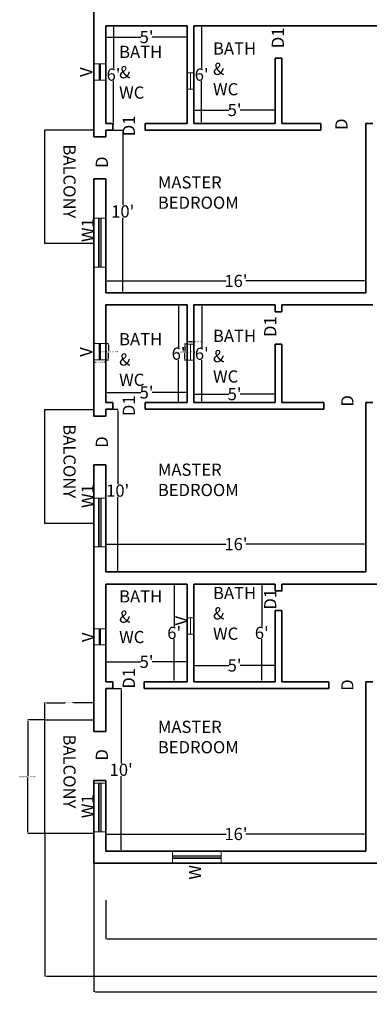
# Model space of a CAD drawing. Units: inches. Extents: x -2189 to 546, y 945 to 2684.
# Tile 1 of 10: x -884 to -626, y 945 to 1672. Entities that reach past the tile are written whole.
import ezdxf

# ---------------------------------------------------------------- set-up
doc = ezdxf.new("R2010")
doc.units = ezdxf.units.IN
doc.header["$MEASUREMENT"] = 0
for name, color, linetype, lineweight in [('A-ANNO-DIMS', 2, 'Continuous', 13), ('A-ANNO-TEXT', 7, 'Continuous', 18), ('A-AREA-IDEN', 3, 'Continuous', 18), ('A-FLOR-BALC', 8, 'Continuous', 25), ('A-GLAZ', 4, 'Continuous', 18), ('A-WALL', 7, 'Continuous', 35)]:
    doc.layers.add(name, color=color, linetype=linetype, lineweight=lineweight)
doc.styles.get("Standard").update_dxf_attribs({"font": 'arial.ttf'})
doc.dimstyles.get("Standard").update_dxf_attribs({"dimtxt": 1, "dimasz": 1, "dimexe": 0.18, "dimexo": 0.0625, "dimgap": 0.09, "dimtad": 0, "dimtih": 1, "dimtoh": 1, "dimdec": 0, "dimzin": 0, "dimdsep": 46, "dimlunit": 3, "dimtxsty": 'Standard', "dimcen": 0.09, "dimadec": 0, "dimazin": 0, "dimtfac": 1, "dimtdec": 0, "dimtofl": 0, "dimtmove": 0, "dimatfit": 3, "dimfxl": 1, "dimtolj": 1, "dimtzin": 0, "dimarcsym": 0})

# ---------------------------------------------------------------- blocks, each defined once
blk = doc.blocks.new('*D1')
at = {"layer": 'A-ANNO-DIMS', "color": 0, "lineweight": -2, "transparency": 16777216}
for p, q in [((-820.72, 1178.17), (-809.35, 1178.17)), ((-809.53, 1177.17), (-809.53, 1122.86)), ((-809.53, 1059.17), (-809.53, 1113.49)), ((-820.72, 1058.17), (-809.35, 1058.17))]:
    blk.add_line(p, q, dxfattribs=at)
at = {"layer": 'A-ANNO-DIMS', "color": 0, "transparency": 16777216}
for points in [[(-809.7, 1177.17), (-809.37, 1177.17), (-809.53, 1178.17)], [(-809.7, 1059.17), (-809.37, 1059.17), (-809.53, 1058.17)]]:
    blk.add_solid(points, dxfattribs=at)
at = {"layer": 'Defpoints', "color": 0, "transparency": 16777216}
for p in [(-820.78, 1178.17), (-820.78, 1058.17), (-809.53, 1058.17)]:
    blk.add_point(p, dxfattribs=at)
at = {"layer": 'A-ANNO-DIMS', "color": 0, "transparency": 16777216, "insert": (-809.53, 1118.17), "char_height": 1, "attachment_point": 5}
blk.add_mtext("\\A1;{\\H9x;10'}", dxfattribs=at)
blk = doc.blocks.new('*D2')
at = {"layer": 'A-ANNO-DIMS', "color": 0, "lineweight": -2, "transparency": 16777216}
for p, q in [((-820.78, 1058.24), (-820.78, 1070.92)), ((-819.78, 1070.74), (-732.08, 1070.74)), ((-629.78, 1070.74), (-717.48, 1070.74)), ((-628.78, 1058.24), (-628.78, 1070.92))]:
    blk.add_line(p, q, dxfattribs=at)
at = {"layer": 'A-ANNO-DIMS', "color": 0, "transparency": 16777216}
for points in [[(-819.78, 1070.9), (-819.78, 1070.57), (-820.78, 1070.74)], [(-629.78, 1070.9), (-629.78, 1070.57), (-628.78, 1070.74)]]:
    blk.add_solid(points, dxfattribs=at)
at = {"layer": 'Defpoints', "color": 0, "transparency": 16777216}
for p in [(-820.78, 1070.74), (-820.78, 1058.17), (-628.78, 1058.17)]:
    blk.add_point(p, dxfattribs=at)
at = {"layer": 'A-ANNO-DIMS', "color": 0, "transparency": 16777216, "insert": (-724.78, 1070.74), "char_height": 1, "attachment_point": 5}
blk.add_mtext("\\A1;{\\H9x;16'}", dxfattribs=at)
blk = doc.blocks.new('*D9')
at = {"layer": 'A-ANNO-DIMS', "color": 0, "lineweight": -2, "transparency": 16777216}
for p, q in [((-760.84, 1255.17), (-770.56, 1255.17)), ((-770.38, 1254.17), (-770.38, 1223.86)), ((-770.38, 1184.17), (-770.38, 1214.49)), ((-760.84, 1183.17), (-770.56, 1183.17))]:
    blk.add_line(p, q, dxfattribs=at)
at = {"layer": 'A-ANNO-DIMS', "color": 0, "transparency": 16777216}
for points in [[(-770.55, 1254.17), (-770.22, 1254.17), (-770.38, 1255.17)], [(-770.55, 1184.17), (-770.22, 1184.17), (-770.38, 1183.17)]]:
    blk.add_solid(points, dxfattribs=at)
at = {"layer": 'Defpoints', "color": 0, "transparency": 16777216}
for p in [(-760.78, 1255.17), (-770.38, 1183.17), (-760.78, 1183.17)]:
    blk.add_point(p, dxfattribs=at)
at = {"layer": 'A-ANNO-DIMS', "color": 0, "transparency": 16777216, "insert": (-770.38, 1219.17), "char_height": 1, "attachment_point": 5}
blk.add_mtext("\\A1;{\\H9x;6'}", dxfattribs=at)
blk = doc.blocks.new('*D10')
at = {"layer": 'A-ANNO-DIMS', "color": 0, "lineweight": -2, "transparency": 16777216}
for p, q in [((-820.78, 1183.24), (-820.78, 1198.02)), ((-819.78, 1197.84), (-795.01, 1197.84)), ((-761.78, 1197.84), (-786.55, 1197.84)), ((-760.78, 1183.24), (-760.78, 1198.02))]:
    blk.add_line(p, q, dxfattribs=at)
at = {"layer": 'A-ANNO-DIMS', "color": 0, "transparency": 16777216}
for points in [[(-819.78, 1198.01), (-819.78, 1197.67), (-820.78, 1197.84)], [(-761.78, 1198.01), (-761.78, 1197.67), (-760.78, 1197.84)]]:
    blk.add_solid(points, dxfattribs=at)
at = {"layer": 'Defpoints', "color": 0, "transparency": 16777216}
for p in [(-760.78, 1197.84), (-820.78, 1183.17), (-760.78, 1183.17)]:
    blk.add_point(p, dxfattribs=at)
at = {"layer": 'A-ANNO-DIMS', "color": 0, "transparency": 16777216, "insert": (-790.78, 1197.84), "char_height": 1, "attachment_point": 5}
blk.add_mtext("\\A1;{\\H9x;5'}", dxfattribs=at)
blk = doc.blocks.new('*D11')
at = {"layer": 'A-ANNO-DIMS', "color": 0, "lineweight": -2, "transparency": 16777216}
for p, q in [((-695.84, 1255.17), (-705.88, 1255.17)), ((-705.7, 1254.17), (-705.7, 1223.86)), ((-705.7, 1184.17), (-705.7, 1214.49)), ((-695.84, 1183.17), (-705.88, 1183.17))]:
    blk.add_line(p, q, dxfattribs=at)
at = {"layer": 'A-ANNO-DIMS', "color": 0, "transparency": 16777216}
for points in [[(-705.87, 1254.17), (-705.53, 1254.17), (-705.7, 1255.17)], [(-705.87, 1184.17), (-705.53, 1184.17), (-705.7, 1183.17)]]:
    blk.add_solid(points, dxfattribs=at)
at = {"layer": 'Defpoints', "color": 0, "transparency": 16777216}
for p in [(-695.78, 1255.17), (-705.7, 1183.17), (-695.78, 1183.17)]:
    blk.add_point(p, dxfattribs=at)
at = {"layer": 'A-ANNO-DIMS', "color": 0, "transparency": 16777216, "insert": (-705.7, 1219.17), "char_height": 1, "attachment_point": 5}
blk.add_mtext("\\A1;{\\H9x;6'}", dxfattribs=at)
blk = doc.blocks.new('*D12')
at = {"layer": 'A-ANNO-DIMS', "color": 0, "lineweight": -2, "transparency": 16777216}
for p, q in [((-755.78, 1183.24), (-755.78, 1195.33)), ((-754.78, 1195.15), (-730.01, 1195.15)), ((-696.78, 1195.15), (-721.55, 1195.15)), ((-695.78, 1183.24), (-695.78, 1195.33))]:
    blk.add_line(p, q, dxfattribs=at)
at = {"layer": 'A-ANNO-DIMS', "color": 0, "transparency": 16777216}
for points in [[(-754.78, 1195.31), (-754.78, 1194.98), (-755.78, 1195.15)], [(-696.78, 1195.31), (-696.78, 1194.98), (-695.78, 1195.15)]]:
    blk.add_solid(points, dxfattribs=at)
at = {"layer": 'Defpoints', "color": 0, "transparency": 16777216}
for p in [(-695.78, 1195.15), (-755.78, 1183.17), (-695.78, 1183.17)]:
    blk.add_point(p, dxfattribs=at)
at = {"layer": 'A-ANNO-DIMS', "color": 0, "transparency": 16777216, "insert": (-725.78, 1195.15), "char_height": 1, "attachment_point": 5}
blk.add_mtext("\\A1;{\\H9x;5'}", dxfattribs=at)
blk = doc.blocks.new('*D13')
at = {"layer": 'A-ANNO-DIMS', "color": 0, "lineweight": -2, "transparency": 16777216}
for p, q in [((-820.78, 1264.24), (-820.78, 1284.87)), ((-819.78, 1284.69), (-732.08, 1284.69)), ((-629.78, 1284.69), (-717.48, 1284.69)), ((-628.78, 1264.24), (-628.78, 1284.87))]:
    blk.add_line(p, q, dxfattribs=at)
at = {"layer": 'A-ANNO-DIMS', "color": 0, "transparency": 16777216}
for points in [[(-819.78, 1284.85), (-819.78, 1284.52), (-820.78, 1284.69)], [(-629.78, 1284.85), (-629.78, 1284.52), (-628.78, 1284.69)]]:
    blk.add_solid(points, dxfattribs=at)
at = {"layer": 'Defpoints', "color": 0, "transparency": 16777216}
for p in [(-628.78, 1284.69), (-820.78, 1264.17), (-628.78, 1264.17)]:
    blk.add_point(p, dxfattribs=at)
at = {"layer": 'A-ANNO-DIMS', "color": 0, "transparency": 16777216, "insert": (-724.78, 1284.69), "char_height": 1, "attachment_point": 5}
blk.add_mtext("\\A1;{\\H9x;16'}", dxfattribs=at)
blk = doc.blocks.new('*D14')
at = {"layer": 'A-ANNO-DIMS', "color": 0, "lineweight": -2, "transparency": 16777216}
for p, q in [((-820.72, 1384.17), (-811.93, 1384.17)), ((-812.11, 1383.17), (-812.11, 1328.86)), ((-812.11, 1265.17), (-812.11, 1319.49)), ((-820.72, 1264.17), (-811.93, 1264.17))]:
    blk.add_line(p, q, dxfattribs=at)
at = {"layer": 'A-ANNO-DIMS', "color": 0, "transparency": 16777216}
for points in [[(-812.28, 1383.17), (-811.94, 1383.17), (-812.11, 1384.17)], [(-812.28, 1265.17), (-811.94, 1265.17), (-812.11, 1264.17)]]:
    blk.add_solid(points, dxfattribs=at)
at = {"layer": 'Defpoints', "color": 0, "transparency": 16777216}
for p in [(-820.78, 1384.17), (-812.11, 1384.17), (-820.78, 1264.17)]:
    blk.add_point(p, dxfattribs=at)
at = {"layer": 'A-ANNO-DIMS', "color": 0, "transparency": 16777216, "insert": (-812.11, 1324.17), "char_height": 1, "attachment_point": 5}
blk.add_mtext("\\A1;{\\H9x;10'}", dxfattribs=at)
blk = doc.blocks.new('*D15')
at = {"layer": 'A-ANNO-DIMS', "color": 0, "lineweight": -2, "transparency": 16777216}
for p, q in [((-820.78, 1389.24), (-820.78, 1396.78)), ((-819.78, 1396.6), (-795.01, 1396.6)), ((-761.78, 1396.6), (-786.55, 1396.6)), ((-760.78, 1389.24), (-760.78, 1396.78))]:
    blk.add_line(p, q, dxfattribs=at)
at = {"layer": 'A-ANNO-DIMS', "color": 0, "transparency": 16777216}
for points in [[(-819.78, 1396.77), (-819.78, 1396.44), (-820.78, 1396.6)], [(-761.78, 1396.77), (-761.78, 1396.44), (-760.78, 1396.6)]]:
    blk.add_solid(points, dxfattribs=at)
at = {"layer": 'Defpoints', "color": 0, "transparency": 16777216}
for p in [(-760.78, 1396.6), (-820.78, 1389.17), (-760.78, 1389.17)]:
    blk.add_point(p, dxfattribs=at)
at = {"layer": 'A-ANNO-DIMS', "color": 0, "transparency": 16777216, "insert": (-790.78, 1396.6), "char_height": 1, "attachment_point": 5}
blk.add_mtext("\\A1;{\\H9x;5'}", dxfattribs=at)
blk = doc.blocks.new('*D16')
at = {"layer": 'A-ANNO-DIMS', "color": 0, "lineweight": -2, "transparency": 16777216}
for p, q in [((-760.84, 1461.17), (-767.31, 1461.17)), ((-767.13, 1460.17), (-767.13, 1429.86)), ((-767.13, 1390.17), (-767.13, 1420.49)), ((-760.84, 1389.17), (-767.31, 1389.17))]:
    blk.add_line(p, q, dxfattribs=at)
at = {"layer": 'A-ANNO-DIMS', "color": 0, "transparency": 16777216}
for points in [[(-767.3, 1460.17), (-766.97, 1460.17), (-767.13, 1461.17)], [(-767.3, 1390.17), (-766.97, 1390.17), (-767.13, 1389.17)]]:
    blk.add_solid(points, dxfattribs=at)
at = {"layer": 'Defpoints', "color": 0, "transparency": 16777216}
for p in [(-767.13, 1461.17), (-760.78, 1461.17), (-760.78, 1389.17)]:
    blk.add_point(p, dxfattribs=at)
at = {"layer": 'A-ANNO-DIMS', "color": 0, "transparency": 16777216, "insert": (-767.13, 1425.17), "char_height": 1, "attachment_point": 5}
blk.add_mtext("\\A1;{\\H9x;6'}", dxfattribs=at)
blk = doc.blocks.new('*D17')
at = {"layer": 'A-ANNO-DIMS', "color": 0, "lineweight": -2, "transparency": 16777216}
for p, q in [((-755.78, 1389.24), (-755.78, 1395.56)), ((-754.78, 1395.38), (-730.01, 1395.38)), ((-696.78, 1395.38), (-721.55, 1395.38)), ((-695.78, 1389.24), (-695.78, 1395.56))]:
    blk.add_line(p, q, dxfattribs=at)
at = {"layer": 'A-ANNO-DIMS', "color": 0, "transparency": 16777216}
for points in [[(-754.78, 1395.55), (-754.78, 1395.21), (-755.78, 1395.38)], [(-696.78, 1395.55), (-696.78, 1395.21), (-695.78, 1395.38)]]:
    blk.add_solid(points, dxfattribs=at)
at = {"layer": 'Defpoints', "color": 0, "transparency": 16777216}
for p in [(-695.78, 1395.38), (-755.78, 1389.17), (-695.78, 1389.17)]:
    blk.add_point(p, dxfattribs=at)
at = {"layer": 'A-ANNO-DIMS', "color": 0, "transparency": 16777216, "insert": (-725.78, 1395.38), "char_height": 1, "attachment_point": 5}
blk.add_mtext("\\A1;{\\H9x;5'}", dxfattribs=at)
blk = doc.blocks.new('*D18')
at = {"layer": 'A-ANNO-DIMS', "color": 0, "lineweight": -2, "transparency": 16777216}
for p, q in [((-755.72, 1461.17), (-749.83, 1461.17)), ((-750.01, 1460.17), (-750.01, 1429.86)), ((-750.01, 1390.17), (-750.01, 1420.49)), ((-755.72, 1389.17), (-749.83, 1389.17))]:
    blk.add_line(p, q, dxfattribs=at)
at = {"layer": 'A-ANNO-DIMS', "color": 0, "transparency": 16777216}
for points in [[(-750.18, 1460.17), (-749.84, 1460.17), (-750.01, 1461.17)], [(-750.18, 1390.17), (-749.84, 1390.17), (-750.01, 1389.17)]]:
    blk.add_solid(points, dxfattribs=at)
at = {"layer": 'Defpoints', "color": 0, "transparency": 16777216}
for p in [(-755.78, 1461.17), (-755.78, 1389.17), (-750.01, 1389.17)]:
    blk.add_point(p, dxfattribs=at)
at = {"layer": 'A-ANNO-DIMS', "color": 0, "transparency": 16777216, "insert": (-750.01, 1425.17), "char_height": 1, "attachment_point": 5}
blk.add_mtext("\\A1;{\\H9x;6'}", dxfattribs=at)
blk = doc.blocks.new('*D25')
at = {"layer": 'A-ANNO-DIMS', "color": 0, "lineweight": -2, "transparency": 16777216}
for p, q in [((-820.78, 1470.24), (-820.78, 1479.07)), ((-819.78, 1478.89), (-732.08, 1478.89)), ((-629.78, 1478.89), (-717.48, 1478.89)), ((-628.78, 1470.24), (-628.78, 1479.07))]:
    blk.add_line(p, q, dxfattribs=at)
at = {"layer": 'A-ANNO-DIMS', "color": 0, "transparency": 16777216}
for points in [[(-819.78, 1479.06), (-819.78, 1478.72), (-820.78, 1478.89)], [(-629.78, 1479.06), (-629.78, 1478.72), (-628.78, 1478.89)]]:
    blk.add_solid(points, dxfattribs=at)
at = {"layer": 'Defpoints', "color": 0, "transparency": 16777216}
for p in [(-628.78, 1478.89), (-820.78, 1470.17), (-628.78, 1470.17)]:
    blk.add_point(p, dxfattribs=at)
at = {"layer": 'A-ANNO-DIMS', "color": 0, "transparency": 16777216, "insert": (-724.78, 1478.89), "char_height": 1, "attachment_point": 5}
blk.add_mtext("\\A1;{\\H9x;16'}", dxfattribs=at)
blk = doc.blocks.new('*D26')
at = {"layer": 'A-ANNO-DIMS', "color": 0, "lineweight": -2, "transparency": 16777216}
for p, q in [((-820.72, 1590.17), (-808.2, 1590.17)), ((-808.38, 1589.17), (-808.38, 1534.86)), ((-808.38, 1471.17), (-808.38, 1525.49)), ((-820.72, 1470.17), (-808.2, 1470.17))]:
    blk.add_line(p, q, dxfattribs=at)
at = {"layer": 'A-ANNO-DIMS', "color": 0, "transparency": 16777216}
for points in [[(-808.55, 1589.17), (-808.22, 1589.17), (-808.38, 1590.17)], [(-808.55, 1471.17), (-808.22, 1471.17), (-808.38, 1470.17)]]:
    blk.add_solid(points, dxfattribs=at)
at = {"layer": 'Defpoints', "color": 0, "transparency": 16777216}
for p in [(-820.78, 1590.17), (-808.38, 1590.17), (-820.78, 1470.17)]:
    blk.add_point(p, dxfattribs=at)
at = {"layer": 'A-ANNO-DIMS', "color": 0, "transparency": 16777216, "insert": (-808.38, 1530.17), "char_height": 1, "attachment_point": 5}
blk.add_mtext("\\A1;{\\H9x;10'}", dxfattribs=at)
blk = doc.blocks.new('*D27')
at = {"layer": 'A-ANNO-DIMS', "color": 0, "lineweight": -2, "transparency": 16777216}
for p, q in [((-820.78, 1667.11), (-820.78, 1658.69)), ((-760.78, 1667.11), (-760.78, 1658.69)), ((-819.78, 1658.87), (-795.01, 1658.87)), ((-761.78, 1658.87), (-786.55, 1658.87))]:
    blk.add_line(p, q, dxfattribs=at)
at = {"layer": 'A-ANNO-DIMS', "color": 0, "transparency": 16777216}
for points in [[(-819.78, 1659.03), (-819.78, 1658.7), (-820.78, 1658.87)], [(-761.78, 1659.03), (-761.78, 1658.7), (-760.78, 1658.87)]]:
    blk.add_solid(points, dxfattribs=at)
at = {"layer": 'Defpoints', "color": 0, "transparency": 16777216}
for p in [(-820.78, 1667.17), (-760.78, 1667.17), (-760.78, 1658.87)]:
    blk.add_point(p, dxfattribs=at)
at = {"layer": 'A-ANNO-DIMS', "color": 0, "transparency": 16777216, "insert": (-790.78, 1658.87), "char_height": 1, "attachment_point": 5}
blk.add_mtext("\\A1;{\\H9x;5'}", dxfattribs=at)
blk = doc.blocks.new('*D28')
at = {"layer": 'A-ANNO-DIMS', "color": 0, "lineweight": -2, "transparency": 16777216}
for p, q in [((-820.72, 1667.17), (-815, 1667.17)), ((-815.18, 1666.17), (-815.18, 1635.86)), ((-815.18, 1596.17), (-815.18, 1626.49)), ((-820.72, 1595.17), (-815, 1595.17))]:
    blk.add_line(p, q, dxfattribs=at)
at = {"layer": 'A-ANNO-DIMS', "color": 0, "transparency": 16777216}
for points in [[(-815.35, 1666.17), (-815.01, 1666.17), (-815.18, 1667.17)], [(-815.35, 1596.17), (-815.01, 1596.17), (-815.18, 1595.17)]]:
    blk.add_solid(points, dxfattribs=at)
at = {"layer": 'Defpoints', "color": 0, "transparency": 16777216}
for p in [(-820.78, 1667.17), (-815.18, 1667.17), (-820.78, 1595.17)]:
    blk.add_point(p, dxfattribs=at)
at = {"layer": 'A-ANNO-DIMS', "color": 0, "transparency": 16777216, "insert": (-815.18, 1631.17), "char_height": 1, "attachment_point": 5}
blk.add_mtext("\\A1;{\\H9x;6'}", dxfattribs=at)
blk = doc.blocks.new('*D29')
at = {"layer": 'A-ANNO-DIMS', "color": 0, "lineweight": -2, "transparency": 16777216}
for p, q in [((-755.78, 1595.24), (-755.78, 1605.21)), ((-754.78, 1605.03), (-730.01, 1605.03)), ((-696.78, 1605.03), (-721.55, 1605.03)), ((-695.78, 1595.24), (-695.78, 1605.21))]:
    blk.add_line(p, q, dxfattribs=at)
at = {"layer": 'A-ANNO-DIMS', "color": 0, "transparency": 16777216}
for points in [[(-754.78, 1605.2), (-754.78, 1604.87), (-755.78, 1605.03)], [(-696.78, 1605.2), (-696.78, 1604.87), (-695.78, 1605.03)]]:
    blk.add_solid(points, dxfattribs=at)
at = {"layer": 'Defpoints', "color": 0, "transparency": 16777216}
for p in [(-695.78, 1605.03), (-755.78, 1595.17), (-695.78, 1595.17)]:
    blk.add_point(p, dxfattribs=at)
at = {"layer": 'A-ANNO-DIMS', "color": 0, "transparency": 16777216, "insert": (-725.78, 1605.03), "char_height": 1, "attachment_point": 5}
blk.add_mtext("\\A1;{\\H9x;5'}", dxfattribs=at)
blk = doc.blocks.new('*D30')
at = {"layer": 'A-ANNO-DIMS', "color": 0, "lineweight": -2, "transparency": 16777216}
for p, q in [((-755.72, 1667.17), (-749.91, 1667.17)), ((-750.09, 1666.17), (-750.09, 1635.86)), ((-750.09, 1596.17), (-750.09, 1626.49)), ((-755.72, 1595.17), (-749.91, 1595.17))]:
    blk.add_line(p, q, dxfattribs=at)
at = {"layer": 'A-ANNO-DIMS', "color": 0, "transparency": 16777216}
for points in [[(-750.26, 1666.17), (-749.93, 1666.17), (-750.09, 1667.17)], [(-750.26, 1596.17), (-749.93, 1596.17), (-750.09, 1595.17)]]:
    blk.add_solid(points, dxfattribs=at)
at = {"layer": 'Defpoints', "color": 0, "transparency": 16777216}
for p in [(-755.78, 1667.17), (-750.09, 1667.17), (-755.78, 1595.17)]:
    blk.add_point(p, dxfattribs=at)
at = {"layer": 'A-ANNO-DIMS', "color": 0, "transparency": 16777216, "insert": (-750.09, 1631.17), "char_height": 1, "attachment_point": 5}
blk.add_mtext("\\A1;{\\H9x;6'}", dxfattribs=at)
blk = doc.blocks.new('*D81')
at = {"layer": 'A-ANNO-DIMS', "color": 0, "lineweight": -2, "transparency": 16777216}
for p, q in [((-829.78, 1049.11), (-829.78, 954.22)), ((-262.78, 1049.11), (-262.78, 954.22)), ((-828.78, 954.4), (-577.65, 954.4)), ((-263.78, 954.4), (-514.91, 954.4))]:
    blk.add_line(p, q, dxfattribs=at)
at = {"layer": 'A-ANNO-DIMS', "color": 0, "transparency": 16777216}
for points in [[(-828.78, 954.57), (-828.78, 954.24), (-829.78, 954.4)], [(-263.78, 954.57), (-263.78, 954.24), (-262.78, 954.4)]]:
    blk.add_solid(points, dxfattribs=at)
at = {"layer": 'Defpoints', "color": 0, "transparency": 16777216}
for p in [(-829.78, 1049.17), (-262.78, 1049.17), (-262.78, 954.4)]:
    blk.add_point(p, dxfattribs=at)
at = {"layer": 'A-ANNO-DIMS', "color": 0, "transparency": 16777216, "insert": (-546.28, 954.4), "char_height": 1, "attachment_point": 5}
blk.add_mtext('\\A1;{\\H18x;47\'-3"}', dxfattribs=at)
blk = doc.blocks.new('*D82')
at = {"layer": 'A-ANNO-DIMS', "color": 0, "lineweight": -2, "transparency": 16777216}
for p, q in [((-820.78, 1021.94), (-820.78, 993.18)), ((-271.78, 1021.94), (-271.78, 993.18)), ((-819.78, 993.36), (-577.65, 993.36)), ((-272.78, 993.36), (-514.91, 993.36))]:
    blk.add_line(p, q, dxfattribs=at)
at = {"layer": 'A-ANNO-DIMS', "color": 0, "transparency": 16777216}
for points in [[(-819.78, 993.52), (-819.78, 993.19), (-820.78, 993.36)], [(-272.78, 993.52), (-272.78, 993.19), (-271.78, 993.36)]]:
    blk.add_solid(points, dxfattribs=at)
at = {"layer": 'Defpoints', "color": 0, "transparency": 16777216}
for p in [(-820.78, 1022), (-271.78, 1022), (-271.78, 993.36)]:
    blk.add_point(p, dxfattribs=at)
at = {"layer": 'A-ANNO-DIMS', "color": 0, "transparency": 16777216, "insert": (-546.28, 993.36), "char_height": 1, "attachment_point": 5}
blk.add_mtext('\\A1;{\\H18x;45\'-9"}', dxfattribs=at)
blk = doc.blocks.new('WIN-36X9')
for p, q in [((0, 5.5), (36, 5.5)), ((0, 5.5), (36, 5.5)), ((0, 4.5), (36, 4.5)), ((0, 3.5), (36, 3.5))]:
    blk.add_line(p, q)
blk.add_lwpolyline([(0, 0), (0, 9), (36, 9), (36, 0)], close=True)
blk = doc.blocks.new('VENT-12X5')
blk.add_line((2.5, 12), (2.5, 0))
blk.add_lwpolyline([(5, 12), (0, 12), (0, 0), (5, 0)], close=True)
blk = doc.blocks.new('VENT-12X9-MULTILINE')
for p, q in [((4, 12), (4, 0)), ((4.5, 12), (4.5, 0)), ((5, 12), (5, 0))]:
    blk.add_line(p, q)
blk.add_lwpolyline([(0, 12), (9, 12), (9, 0), (0, 0)], close=True)
blk = doc.blocks.new('BALCONY-36X84')
for p, q in [((0, 0), (0, 84)), ((0, 84), (36, 84)), ((36, 0), (0, 0))]:
    blk.add_line(p, q)
blk = doc.blocks.new('*D95')
at = {"layer": 'A-ANNO-DIMS', "color": 0, "lineweight": -2, "transparency": 16777216}
for p, q in [((-760.84, 1432.3), (-762.76, 1432.3)), ((-762.58, 1431.3), (-762.58, 1426.91)), ((-762.58, 1421.3), (-762.58, 1425.69)), ((-760.84, 1420.3), (-762.76, 1420.3))]:
    blk.add_line(p, q, dxfattribs=at)
at = {"layer": 'A-ANNO-DIMS', "color": 0, "transparency": 16777216}
for points in [[(-762.75, 1431.3), (-762.41, 1431.3), (-762.58, 1432.3)], [(-762.75, 1421.3), (-762.41, 1421.3), (-762.58, 1420.3)]]:
    blk.add_solid(points, dxfattribs=at)
at = {"layer": 'Defpoints', "color": 0, "transparency": 16777216}
for p in [(-762.58, 1432.3), (-760.78, 1432.3), (-760.78, 1420.3)]:
    blk.add_point(p, dxfattribs=at)
at = {"layer": 'A-ANNO-DIMS', "color": 0, "transparency": 16777216, "insert": (-762.58, 1426.3), "char_height": 1, "attachment_point": 5}
blk.add_mtext('\\A1;PARTITION VENT 1\'-0" TYP.', dxfattribs=at)
blk = doc.blocks.new('*D96')
at = {"layer": 'A-ANNO-DIMS', "color": 0, "lineweight": -2, "transparency": 16777216}
for p, q in [((-760.78, 1432.36), (-760.78, 1434.28)), ((-759.78, 1434.1), (-756.78, 1434.1)), ((-755.78, 1432.36), (-755.78, 1434.28)), ((-755.78, 1434.1), (-754.78, 1434.1))]:
    blk.add_line(p, q, dxfattribs=at)
at = {"layer": 'A-ANNO-DIMS', "color": 0, "transparency": 16777216}
for points in [[(-759.78, 1434.27), (-759.78, 1433.93), (-760.78, 1434.1)], [(-756.78, 1434.27), (-756.78, 1433.93), (-755.78, 1434.1)]]:
    blk.add_solid(points, dxfattribs=at)
at = {"layer": 'Defpoints', "color": 0, "transparency": 16777216}
for p in [(-760.78, 1432.3), (-755.78, 1434.1), (-755.78, 1432.3)]:
    blk.add_point(p, dxfattribs=at)
at = {"layer": 'A-ANNO-DIMS', "color": 0, "transparency": 16777216, "insert": (-751.64, 1434.1), "char_height": 1, "attachment_point": 5}
blk.add_mtext('\\A1;0\'-5" TYP.', dxfattribs=at)
blk = doc.blocks.new('*D99')
at = {"layer": 'A-ANNO-DIMS', "color": 0, "lineweight": -2, "transparency": 16777216}
for p, q in [((-820.72, 1432.67), (-818.8, 1432.67)), ((-818.98, 1431.67), (-818.98, 1427.41)), ((-818.98, 1421.67), (-818.98, 1425.92)), ((-820.72, 1420.67), (-818.8, 1420.67))]:
    blk.add_line(p, q, dxfattribs=at)
at = {"layer": 'A-ANNO-DIMS', "color": 0, "transparency": 16777216}
for points in [[(-819.15, 1431.67), (-818.81, 1431.67), (-818.98, 1432.67)], [(-819.15, 1421.67), (-818.81, 1421.67), (-818.98, 1420.67)]]:
    blk.add_solid(points, dxfattribs=at)
at = {"layer": 'Defpoints', "color": 0, "transparency": 16777216}
for p in [(-820.78, 1432.67), (-818.98, 1432.67), (-820.78, 1420.67)]:
    blk.add_point(p, dxfattribs=at)
at = {"layer": 'A-ANNO-DIMS', "color": 0, "transparency": 16777216, "insert": (-818.98, 1426.67), "char_height": 1, "attachment_point": 5}
blk.add_mtext('\\A1;VENT (MULTI) 1\'-0" TYP.', dxfattribs=at)
blk = doc.blocks.new('*D100')
at = {"layer": 'A-ANNO-DIMS', "color": 0, "lineweight": -2, "transparency": 16777216}
for p, q in [((-829.78, 1420.6), (-829.78, 1418.69)), ((-828.78, 1418.87), (-828.42, 1418.87)), ((-821.78, 1418.87), (-822.14, 1418.87)), ((-820.78, 1420.6), (-820.78, 1418.69))]:
    blk.add_line(p, q, dxfattribs=at)
at = {"layer": 'A-ANNO-DIMS', "color": 0, "transparency": 16777216}
for points in [[(-828.78, 1419.03), (-828.78, 1418.7), (-829.78, 1418.87)], [(-821.78, 1419.03), (-821.78, 1418.7), (-820.78, 1418.87)]]:
    blk.add_solid(points, dxfattribs=at)
at = {"layer": 'Defpoints', "color": 0, "transparency": 16777216}
for p in [(-829.78, 1420.67), (-820.78, 1420.67), (-820.78, 1418.87)]:
    blk.add_point(p, dxfattribs=at)
at = {"layer": 'A-ANNO-DIMS', "color": 0, "transparency": 16777216, "insert": (-825.28, 1418.87), "char_height": 1, "attachment_point": 5}
blk.add_mtext('\\A1;0\'-9" TYP.', dxfattribs=at)
blk = doc.blocks.new('*D101')
at = {"layer": 'A-ANNO-DIMS', "color": 0, "lineweight": -2, "transparency": 16777216}
for p, q in [((-865.84, 1155.01), (-878.56, 1155.01)), ((-878.38, 1154.01), (-878.38, 1113.61)), ((-878.38, 1072.01), (-878.38, 1112.4)), ((-865.84, 1071.01), (-878.56, 1071.01))]:
    blk.add_line(p, q, dxfattribs=at)
at = {"layer": 'A-ANNO-DIMS', "color": 0, "transparency": 16777216}
for points in [[(-878.55, 1154.01), (-878.21, 1154.01), (-878.38, 1155.01)], [(-878.55, 1072.01), (-878.21, 1072.01), (-878.38, 1071.01)]]:
    blk.add_solid(points, dxfattribs=at)
at = {"layer": 'Defpoints', "color": 0, "transparency": 16777216}
for p in [(-878.38, 1155.01), (-865.78, 1155.01), (-865.78, 1071.01)]:
    blk.add_point(p, dxfattribs=at)
at = {"layer": 'A-ANNO-DIMS', "color": 0, "transparency": 16777216, "insert": (-878.38, 1113.01), "char_height": 1, "attachment_point": 5}
blk.add_mtext('\\A1;BALCONY 7\'-0" TYP.', dxfattribs=at)
blk = doc.blocks.new('*D102')
at = {"layer": 'A-ANNO-DIMS', "color": 0, "lineweight": -2, "transparency": 16777216}
for p, q in [((-865.78, 1155.07), (-865.78, 1167.79)), ((-864.78, 1167.61), (-850.92, 1167.61)), ((-830.78, 1167.61), (-844.64, 1167.61)), ((-829.78, 1155.07), (-829.78, 1167.79))]:
    blk.add_line(p, q, dxfattribs=at)
at = {"layer": 'A-ANNO-DIMS', "color": 0, "transparency": 16777216}
for points in [[(-864.78, 1167.77), (-864.78, 1167.44), (-865.78, 1167.61)], [(-830.78, 1167.77), (-830.78, 1167.44), (-829.78, 1167.61)]]:
    blk.add_solid(points, dxfattribs=at)
at = {"layer": 'Defpoints', "color": 0, "transparency": 16777216}
for p in [(-829.78, 1167.61), (-865.78, 1155.01), (-829.78, 1155.01)]:
    blk.add_point(p, dxfattribs=at)
at = {"layer": 'A-ANNO-DIMS', "color": 0, "transparency": 16777216, "insert": (-847.78, 1167.61), "char_height": 1, "attachment_point": 5}
blk.add_mtext('\\A1;3\'-0" TYP.', dxfattribs=at)
blk = doc.blocks.new('*D103')
at = {"layer": 'A-ANNO-DIMS', "color": 0, "lineweight": -2, "transparency": 16777216}
for p, q in [((-865.78, 1070.94), (-865.78, 965.69)), ((-262.78, 1049.11), (-262.78, 965.69)), ((-864.78, 965.87), (-566.09, 965.87)), ((-263.78, 965.87), (-562.47, 965.87))]:
    blk.add_line(p, q, dxfattribs=at)
at = {"layer": 'A-ANNO-DIMS', "color": 0, "transparency": 16777216}
for points in [[(-864.78, 966.04), (-864.78, 965.71), (-865.78, 965.87)], [(-263.78, 966.04), (-263.78, 965.71), (-262.78, 965.87)]]:
    blk.add_solid(points, dxfattribs=at)
at = {"layer": 'Defpoints', "color": 0, "transparency": 16777216}
for p in [(-865.78, 1071.01), (-262.78, 1049.17), (-262.78, 965.87)]:
    blk.add_point(p, dxfattribs=at)
at = {"layer": 'A-ANNO-DIMS', "color": 0, "transparency": 16777216, "insert": (-564.28, 965.87), "char_height": 1, "attachment_point": 5}
blk.add_mtext('\\A1;50\'-3"', dxfattribs=at)

msp = doc.modelspace()

# ---------------------------------------------------------------- linework, layer by layer
at = {"layer": 'A-WALL'}
for p, q in [((-829.78, 1585.17), (-829.78, 1755.17)), ((-760.78, 1667.17), (-820.78, 1667.17)), ((-820.78, 1595.17), (-820.78, 1667.17)), ((-760.78, 1595.17), (-760.78, 1667.17)), ((-755.78, 1595.17), (-755.78, 1667.17)), ((-695.78, 1667.17), (-755.78, 1667.17)), ((-366.78, 1667.17), (-695.78, 1667.17)), ((-695.78, 1595.17), (-695.78, 1643.17)), ((-690.78, 1643.17), (-695.78, 1643.17)), ((-690.78, 1595.17), (-690.78, 1643.17)), ((-815.78, 1595.17), (-820.78, 1595.17)), ((-815.78, 1590.17), (-815.78, 1595.17)), ((-760.78, 1595.17), (-791.78, 1595.17)), ((-791.78, 1590.17), (-791.78, 1595.17)), ((-695.78, 1595.17), (-755.78, 1595.17)), ((-662.17, 1595.17), (-690.78, 1595.17)), ((-662.17, 1595.17), (-662.17, 1590.17)), ((-628.78, 1470.17), (-628.78, 1595.17)), ((-623.78, 1595.17), (-628.78, 1595.17)), ((-820.78, 1585.17), (-829.78, 1585.17)), ((-820.78, 1585.17), (-820.78, 1590.17)), ((-815.78, 1590.17), (-820.78, 1590.17)), ((-662.17, 1590.17), (-791.78, 1590.17)), ((-690.78, 1590.17), (-755.78, 1590.17)), ((-662.17, 1590.17), (-690.78, 1590.17)), ((-829.78, 1379.17), (-829.78, 1554.17)), ((-820.78, 1554.17), (-829.78, 1554.17)), ((-820.78, 1470.17), (-820.78, 1554.17)), ((-755.78, 1470.17), (-820.78, 1470.17)), ((-690.78, 1470.17), (-755.78, 1470.17)), ((-628.78, 1470.17), (-690.78, 1470.17)), ((-820.78, 1389.17), (-820.78, 1461.17)), ((-760.78, 1461.17), (-820.78, 1461.17)), ((-760.78, 1389.17), (-760.78, 1461.17)), ((-755.78, 1389.17), (-755.78, 1461.17)), ((-695.78, 1461.17), (-755.78, 1461.17)), ((-695.78, 1456.17), (-695.78, 1461.17)), ((-623.78, 1461.17), (-690.78, 1461.17)), ((-690.78, 1456.17), (-690.78, 1461.17)), ((-695.78, 1456.17), (-690.78, 1456.17)), ((-695.78, 1389.17), (-695.78, 1432.17)), ((-695.78, 1432.17), (-690.78, 1432.17)), ((-690.78, 1389.17), (-690.78, 1432.17)), ((-815.78, 1389.17), (-820.78, 1389.17)), ((-815.78, 1389.17), (-815.78, 1384.17)), ((-760.78, 1389.17), (-791.78, 1389.17)), ((-791.78, 1389.17), (-791.78, 1384.17)), ((-695.78, 1389.17), (-755.78, 1389.17)), ((-659.78, 1389.17), (-690.78, 1389.17)), ((-659.78, 1389.17), (-659.78, 1384.17)), ((-628.78, 1264.17), (-628.78, 1389.17)), ((-623.78, 1389.17), (-628.78, 1389.17)), ((-820.78, 1379.17), (-820.78, 1384.17)), ((-815.78, 1384.17), (-820.78, 1384.17)), ((-659.78, 1384.17), (-791.78, 1384.17)), ((-820.78, 1379.17), (-829.78, 1379.17)), ((-829.78, 1146.35), (-829.78, 1343.17)), ((-820.78, 1343.17), (-829.78, 1343.17)), ((-820.78, 1264.17), (-820.78, 1343.17)), ((-628.78, 1264.17), (-820.78, 1264.17)), ((-820.78, 1183.17), (-820.78, 1255.17)), ((-760.78, 1255.17), (-820.78, 1255.17)), ((-760.78, 1183.17), (-760.78, 1255.17)), ((-755.78, 1183.17), (-755.78, 1255.17)), ((-695.78, 1255.17), (-755.78, 1255.17)), ((-366.78, 1255.17), (-690.78, 1255.17)), ((-695.78, 1183.17), (-695.78, 1235.61)), ((-695.78, 1235.61), (-690.78, 1235.61)), ((-690.78, 1183.17), (-690.78, 1235.61)), ((-820.78, 1146.35), (-820.78, 1178.17)), ((-792.67, 1183.17), (-792.67, 1178.17)), ((-760.78, 1183.17), (-792.67, 1183.17)), ((-656.18, 1178.17), (-792.67, 1178.17)), ((-695.78, 1183.17), (-755.78, 1183.17)), ((-656.18, 1183.17), (-690.78, 1183.17)), ((-656.18, 1178.17), (-656.18, 1183.17)), ((-623.78, 1183.17), (-628.78, 1183.17)), ((-628.78, 1178.17), (-628.78, 1183.17)), ((-628.78, 1058.17), (-628.78, 1178.17)), ((-829.78, 1146.35), (-820.78, 1146.35)), ((-829.78, 1049.17), (-829.78, 1110.35)), ((-829.78, 1110.35), (-820.78, 1110.35)), ((-820.78, 1058.17), (-820.78, 1110.35)), ((-628.78, 1058.17), (-820.78, 1058.17)), ((-262.78, 1049.17), (-829.78, 1049.17))]:
    msp.add_line(p, q, dxfattribs=at)
for points in [[(-695.78, 1255.17), (-695.78, 1250.17), (-690.78, 1250.17), (-690.78, 1255.17)], [(-820.78, 1178.17), (-815.78, 1178.17), (-815.78, 1183.17), (-820.78, 1183.17)]]:
    msp.add_lwpolyline(points, dxfattribs=at)

# ---------------------------------------------------------------- block references
at = {"layer": 'A-FLOR-BALC'}
for p in [(-865.78, 1506.43), (-865.78, 1299.92), (-865.78, 1071.01)]:
    msp.add_blockref('BALCONY-36X84', p, dxfattribs=at)
at = {"layer": 'A-GLAZ'}
for name, p in [('VENT-12X9-MULTILINE', (-829.78, 1627.17)), ('VENT-12X5', (-760.78, 1620.42)), ('VENT-12X9-MULTILINE', (-829.78, 1420.67)), ('VENT-12X5', (-760.78, 1420.3)), ('VENT-12X5', (-760.78, 1218.17)), ('VENT-12X9-MULTILINE', (-829.78, 1210.26)), ('WIN-36X9', (-771.61, 1049.17))]:
    msp.add_blockref(name, p, dxfattribs=at)
for p, rotation in [((-820.78, 1489.16), 90.00000000000142), ((-820.78, 1282.66), 90.0000000000011), ((-820.78, 1072.25), 90.0000000000011)]:
    msp.add_blockref('WIN-36X9', p, dxfattribs=dict(at, rotation=rotation))

# ---------------------------------------------------------------- texts
at = {"layer": 'A-ANNO-TEXT', "char_height": 9, "attachment_point": 1, "rotation": 90}
for s, width, insert in [('D1', 15.3658, (-698.32, 1650.64)), ('V', 17.5973, (-839.88, 1629.43)), ('D1', 15.3658, (-808.38, 1585.67)), ('D', 15.3658, (-651.37, 1590.32)), ('D', 15.3658, (-828.29, 1562.27)), ('W1', 11.3125, (-838.78, 1507.6)), ('D1', 15.3658, (-703.95, 1437.53)), ('V', 17.5973, (-839.88, 1422.92)), ('D1', 15.3658, (-808.38, 1379.16)), ('D', 15.3658, (-646.99, 1386.16)), ('D', 15.3658, (-828.29, 1355.76)), ('W1', 11.3125, (-838.78, 1311.33)), ('D1', 15.3658, (-703.95, 1236.35)), ('V', 17.5973, (-769.56, 1224.62)), ('V', 17.5973, (-838.56, 1212.37)), ('D1', 15.3658, (-808.38, 1177.99)), ('D', 15.3658, (-646.99, 1176.44)), ('D', 15.3658, (-828.29, 1124.97)), ('W1', 11.3125, (-838.78, 1082.42)), ('W', 11.3125, (-759.55, 1037.08))]:
    msp.add_mtext_dynamic_manual_height_columns(s, width=width, gutter_width=1, heights=[0], dxfattribs=dict(at, insert=insert))
at = {"layer": 'A-AREA-IDEN', "char_height": 9, "attachment_point": 1}
for s, width, insert in [('BATH \\P& \\PWC', 29.3144, (-811.04, 1652.41)), ('BATH \\P& \\PWC', 29.3144, (-741.71, 1654.89)), ('MASTER BEDROOM', 73.5764, (-782.43, 1556.12)), ('BATH \\P& \\PWC', 29.3144, (-811.04, 1440.4)), ('BATH \\P& \\PWC', 29.3144, (-741.71, 1442.88)), ('MASTER BEDROOM', 73.5764, (-782.43, 1344.11)), ('BATH \\P& \\PWC', 29.3144, (-811.04, 1250.6)), ('BATH \\P& \\PWC', 29.3144, (-741.71, 1253.09)), ('MASTER BEDROOM', 73.5764, (-782.43, 1154.31))]:
    msp.add_mtext_dynamic_manual_height_columns(s, width=width, gutter_width=1, heights=[0], dxfattribs=dict(at, insert=insert))
at = {"layer": 'A-AREA-IDEN', "char_height": 9, "attachment_point": 1, "rotation": 270}
for insert in [(-843.17, 1579.61), (-843.17, 1373.1), (-843.17, 1144.19)]:
    msp.add_mtext_dynamic_manual_height_columns('BALCONY', width=7.0599, gutter_width=1, heights=[0], dxfattribs=dict(at, insert=insert))

# ---------------------------------------------------------------- dimensions: what is measured, and where the dimension line sits
at = {"layer": 'A-ANNO-DIMS'}
for base, p1, p2, angle, text, override, picture, middle in [((-760.78, 1658.87), (-820.78, 1667.17), (-760.78, 1667.17), 180, '{\\H9x;<>}', {"dimclrd": 0, "dimclre": 0, "dimclrt": 0}, '*D27', (-790.78, 1658.87)), ((-815.18, 1667.17), (-820.78, 1595.17), (-820.78, 1667.17), 90, '{\\H9x;<>}', {"dimclrd": 0, "dimclre": 0, "dimclrt": 0}, '*D28', (-815.18, 1631.17)), ((-750.09, 1667.17), (-755.78, 1595.17), (-755.78, 1667.17), 90, '{\\H9x;<>}', {"dimclrd": 0, "dimclre": 0, "dimclrt": 0}, '*D30', (-750.09, 1631.17)), ((-695.78, 1605.03), (-755.78, 1595.17), (-695.78, 1595.17), 180, '{\\H9x;<>}', {"dimclrd": 0, "dimclre": 0, "dimclrt": 0}, '*D29', (-725.78, 1605.03)), ((-808.38, 1590.17), (-820.78, 1470.17), (-820.78, 1590.17), 90, '{\\H9x;<>}', {"dimclrd": 0, "dimclre": 0, "dimclrt": 0}, '*D26', (-808.38, 1530.17)), ((-628.78, 1478.89), (-820.78, 1470.17), (-628.78, 1470.17), 180, '{\\H9x;<>}', {"dimclrd": 0, "dimclre": 0, "dimclrt": 0}, '*D25', (-724.78, 1478.89)), ((-767.13, 1461.17), (-760.78, 1389.17), (-760.78, 1461.17), 90, '{\\H9x;<>}', {"dimclrd": 0, "dimclre": 0, "dimclrt": 0}, '*D16', (-767.13, 1425.17)), ((-750.01, 1389.17), (-755.78, 1461.17), (-755.78, 1389.17), 90, '{\\H9x;<>}', {"dimclrd": 0, "dimclre": 0, "dimclrt": 0}, '*D18', (-750.01, 1425.17)), ((-818.98, 1432.67), (-820.78, 1420.67), (-820.78, 1432.67), 90, 'VENT (MULTI) <> TYP.', {"dimdec": 1, "dimlfac": 1, "dimrnd": 0, "dimzin": 1, "dimdsep": 46, "dimlunit": 4, "dimfrac": 2}, '*D99', (-818.98, 1426.67)), ((-762.58, 1432.3), (-760.78, 1420.3), (-760.78, 1432.3), 90, 'PARTITION VENT <> TYP.', {"dimdec": 1, "dimlfac": 1, "dimrnd": 0, "dimzin": 1, "dimdsep": 46, "dimlunit": 4, "dimfrac": 2}, '*D95', (-762.58, 1426.3)), ((-760.78, 1396.6), (-820.78, 1389.17), (-760.78, 1389.17), 180, '{\\H9x;<>}', {"dimclrd": 0, "dimclre": 0, "dimclrt": 0}, '*D15', (-790.78, 1396.6)), ((-695.78, 1395.38), (-755.78, 1389.17), (-695.78, 1389.17), 180, '{\\H9x;<>}', {"dimclrd": 0, "dimclre": 0, "dimclrt": 0}, '*D17', (-725.78, 1395.38)), ((-812.11, 1384.17), (-820.78, 1264.17), (-820.78, 1384.17), 90, '{\\H9x;<>}', {"dimclrd": 0, "dimclre": 0, "dimclrt": 0}, '*D14', (-812.11, 1324.17)), ((-628.78, 1284.69), (-820.78, 1264.17), (-628.78, 1264.17), 180, '{\\H9x;<>}', {"dimclrd": 0, "dimclre": 0, "dimclrt": 0}, '*D13', (-724.78, 1284.69)), ((-770.38, 1183.17), (-760.78, 1255.17), (-760.78, 1183.17), 90, '{\\H9x;<>}', {"dimclrd": 0, "dimclre": 0, "dimclrt": 0}, '*D9', (-770.38, 1219.17)), ((-705.7, 1183.17), (-695.78, 1255.17), (-695.78, 1183.17), 90, '{\\H9x;<>}', {"dimclrd": 0, "dimclre": 0, "dimclrt": 0}, '*D11', (-705.7, 1219.17)), ((-809.53, 1058.17), (-820.78, 1178.17), (-820.78, 1058.17), 90, '{\\H9x;<>}', {"dimclrd": 0, "dimclre": 0, "dimclrt": 0}, '*D1', (-809.53, 1118.17)), ((-878.38, 1155.01), (-865.78, 1071.01), (-865.78, 1155.01), 90, 'BALCONY <> TYP.', {"dimdec": 1, "dimlfac": 1, "dimrnd": 0, "dimzin": 1, "dimdsep": 46, "dimlunit": 4, "dimfrac": 2}, '*D101', (-878.38, 1113.01))]:
    dim = msp.add_linear_dim(base=base, p1=p1, p2=p2, angle=angle, text=text, dimstyle='Standard', override=override, dxfattribs=at)
    dim.commit()
    dim.dimension.update_dxf_attribs({"geometry": picture, "text_midpoint": middle})
for base, p1, p2, text, override, picture, middle in [((-755.78, 1434.1), (-760.78, 1432.3), (-755.78, 1432.3), '<> TYP.', {"dimdec": 1, "dimlfac": 1, "dimrnd": 0, "dimzin": 1, "dimdsep": 46, "dimlunit": 4, "dimfrac": 2}, '*D96', (-751.64, 1434.1)), ((-820.78, 1418.87), (-829.78, 1420.67), (-820.78, 1420.67), '<> TYP.', {"dimdec": 1, "dimlfac": 1, "dimrnd": 0, "dimzin": 1, "dimdsep": 46, "dimlunit": 4, "dimfrac": 2}, '*D100', (-825.28, 1418.87)), ((-760.78, 1197.84), (-820.78, 1183.17), (-760.78, 1183.17), '{\\H9x;<>}', {"dimclrd": 0, "dimclre": 0, "dimclrt": 0}, '*D10', (-790.78, 1197.84)), ((-695.78, 1195.15), (-755.78, 1183.17), (-695.78, 1183.17), '{\\H9x;<>}', {"dimclrd": 0, "dimclre": 0, "dimclrt": 0}, '*D12', (-725.78, 1195.15)), ((-829.78, 1167.61), (-865.78, 1155.01), (-829.78, 1155.01), '<> TYP.', {"dimdec": 1, "dimlfac": 1, "dimrnd": 0, "dimzin": 1, "dimdsep": 46, "dimlunit": 4, "dimfrac": 2}, '*D102', (-847.78, 1167.61)), ((-820.78, 1070.74), (-628.78, 1058.17), (-820.78, 1058.17), '{\\H9x;<>}', {"dimclrd": 0, "dimclre": 0, "dimclrt": 0}, '*D2', (-724.78, 1070.74)), ((-262.78, 954.4), (-829.78, 1049.17), (-262.78, 1049.17), '{\\H18x;<>}', {"dimclrd": 0, "dimclre": 0, "dimclrt": 0}, '*D81', (-546.28, 954.4)), ((-271.78, 993.36), (-820.78, 1022), (-271.78, 1022), '{\\H18x;<>}', {"dimclrd": 0, "dimclre": 0, "dimclrt": 0}, '*D82', (-546.28, 993.36))]:
    dim = msp.add_linear_dim(base=base, p1=p1, p2=p2, text=text, dimstyle='Standard', override=override, dxfattribs=at)
    dim.commit()
    dim.dimension.update_dxf_attribs({"geometry": picture, "text_midpoint": middle})
dim = msp.add_linear_dim(base=(-262.78, 965.87), p1=(-865.78, 1071.01), p2=(-262.78, 1049.17), dimstyle='Standard', override={"dimdec": 1, "dimlfac": 1, "dimrnd": 0, "dimzin": 1, "dimdsep": 46, "dimlunit": 4, "dimfrac": 2}, dxfattribs=at)
dim.commit()
dim.dimension.update_dxf_attribs({"geometry": '*D103', "text_midpoint": (-564.28, 965.87)})

doc.saveas('drawing.dxf')
